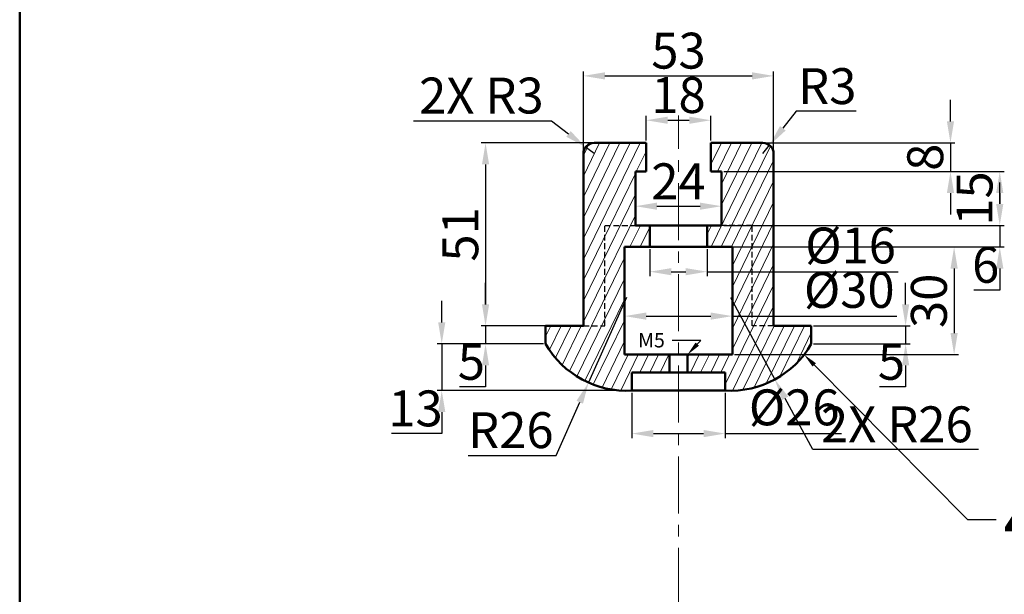
# Model space of a CAD drawing. Units: millimetres. Extents: x 147 to 984, y -369 to 435.
# Tile 2 of 10: x 147 to 422, y -208 to -48. Entities that reach past the tile are written whole.
import ezdxf
from ezdxf import colors
from ezdxf.entities.mleader import LeaderData, LeaderLine
from ezdxf.math import Vec2, Vec3

# ---------------------------------------------------------------- set-up
doc = ezdxf.new("R2010")
doc.units = ezdxf.units.MM
doc.header["$LTSCALE"] = 0.5
doc.linetypes.add('CENTER', pattern=[50.8, 31.75, -6.35, 6.35, -6.35])
doc.linetypes.add('HIDDEN', pattern=[9.525, 6.35, -3.175])
for name, color, linetype, lineweight in [('M-CNTR', 1, 'CENTER', 18), ('M-DIMS', 2, 'Continuous', 25), ('M-HATC', 8, 'Continuous', 18), ('M-HIDN', 3, 'HIDDEN', 25), ('M-OUTL', 7, 'Continuous', 50), ('M-TEXT', 7, 'Continuous', 25)]:
    doc.layers.add(name, color=color, linetype=linetype, lineweight=lineweight)
doc.styles.get("Standard").update_dxf_attribs({"font": 'arial.ttf'})
doc.dimstyles.new('ISO-25', dxfattribs={"dimtxt": 10, "dimasz": 6, "dimexe": 1.25, "dimexo": 0.625, "dimtad": 1, "dimtoh": 1, "dimdec": 0, "dimtxsty": 'Standard', "dimcen": 2.5, "dimadec": 0, "dimazin": 0, "dimtfac": 1, "dimtdec": 0, "dimtmove": 0, "dimatfit": 3, "dimfxl": 1, "dimarcsym": 0})

# ---------------------------------------------------------------- blocks, each defined once
blk = doc.blocks.new('*U94')
at = {"layer": 'M-CNTR', "color": 0, "transparency": 16777216}
blk.add_line((0, -186.27), (0, 51.67), dxfattribs=at)
blk = doc.blocks.new('*D95')
at = {"layer": 'Defpoints', "color": 0, "ltscale": 0.5, "transparency": 16777216}
for p in [(318.85, -100.29), (342.85, -100.29), (342.85, -100.29)]:
    blk.add_point(p, dxfattribs=at)
at = {"layer": 'M-DIMS', "color": 0, "lineweight": -2, "ltscale": 0.5, "transparency": 16777216}
for p, q in [((318.85, -99.67), (318.85, -99.04)), ((324.85, -100.29), (336.85, -100.29)), ((342.85, -99.67), (342.85, -99.04))]:
    blk.add_line(p, q, dxfattribs=at)
at = {"layer": 'M-DIMS', "color": 0, "ltscale": 0.5, "transparency": 16777216}
for points in [[(324.85, -99.29), (324.85, -101.29), (318.85, -100.29)], [(336.85, -99.29), (336.85, -101.29), (342.85, -100.29)]]:
    blk.add_solid(points, dxfattribs=at)
at = {"layer": 'M-DIMS', "color": 0, "ltscale": 0.5, "transparency": 16777216, "insert": (330.85, -94.65), "char_height": 10, "attachment_point": 5}
blk.add_mtext('24', dxfattribs=at)
blk = doc.blocks.new('*D96')
at = {"layer": 'Defpoints', "color": 0, "ltscale": 0.5, "transparency": 16777216}
for p in [(339.85, -76.35), (321.85, -82.65), (339.85, -82.65)]:
    blk.add_point(p, dxfattribs=at)
at = {"layer": 'M-DIMS', "color": 0, "lineweight": -2, "ltscale": 0.5, "transparency": 16777216}
for p, q in [((321.85, -82.03), (321.85, -75.1)), ((327.85, -76.35), (333.85, -76.35)), ((339.85, -82.03), (339.85, -75.1))]:
    blk.add_line(p, q, dxfattribs=at)
at = {"layer": 'M-DIMS', "color": 0, "ltscale": 0.5, "transparency": 16777216}
for points in [[(327.85, -75.35), (327.85, -77.35), (321.85, -76.35)], [(333.85, -75.35), (333.85, -77.35), (339.85, -76.35)]]:
    blk.add_solid(points, dxfattribs=at)
at = {"layer": 'M-DIMS', "color": 0, "ltscale": 0.5, "transparency": 16777216, "insert": (330.85, -70.62), "char_height": 10, "attachment_point": 5}
blk.add_mtext('18', dxfattribs=at)
blk = doc.blocks.new('*D97')
at = {"layer": 'Defpoints', "color": 0, "ltscale": 0.5, "transparency": 16777216}
for p in [(357.35, -63.98), (304.35, -85.65), (357.35, -85.65)]:
    blk.add_point(p, dxfattribs=at)
at = {"layer": 'M-DIMS', "color": 0, "lineweight": -2, "ltscale": 0.5, "transparency": 16777216}
for p, q in [((304.35, -85.03), (304.35, -62.73)), ((357.35, -85.03), (357.35, -62.73)), ((310.35, -63.98), (351.35, -63.98))]:
    blk.add_line(p, q, dxfattribs=at)
at = {"layer": 'M-DIMS', "color": 0, "ltscale": 0.5, "transparency": 16777216}
for points in [[(310.35, -62.98), (310.35, -64.98), (304.35, -63.98)], [(351.35, -62.98), (351.35, -64.98), (357.35, -63.98)]]:
    blk.add_solid(points, dxfattribs=at)
at = {"layer": 'M-DIMS', "color": 0, "ltscale": 0.5, "transparency": 16777216, "insert": (330.85, -58.25), "char_height": 10, "attachment_point": 5}
blk.add_mtext('53', dxfattribs=at)
blk = doc.blocks.new('*D99')
at = {"layer": 'Defpoints', "color": 0, "ltscale": 0.5, "transparency": 16777216}
for p in [(314.6, -82.65), (277.11, -133.65), (299.1, -133.65)]:
    blk.add_point(p, dxfattribs=at)
at = {"layer": 'M-DIMS', "color": 0, "lineweight": -2, "ltscale": 0.5, "transparency": 16777216}
for p, q in [((313.97, -82.65), (275.86, -82.65)), ((277.11, -88.65), (277.11, -127.65)), ((298.47, -133.65), (275.86, -133.65))]:
    blk.add_line(p, q, dxfattribs=at)
at = {"layer": 'M-DIMS', "color": 0, "ltscale": 0.5, "transparency": 16777216}
for points in [[(276.11, -88.65), (278.11, -88.65), (277.11, -82.65)], [(276.11, -127.65), (278.11, -127.65), (277.11, -133.65)]]:
    blk.add_solid(points, dxfattribs=at)
at = {"layer": 'M-DIMS', "color": 0, "ltscale": 0.5, "transparency": 16777216, "insert": (271.37, -108.15), "char_height": 10, "attachment_point": 5, "rotation": 90}
blk.add_mtext('51', dxfattribs=at)
blk = doc.blocks.new('*D100')
at = {"layer": 'Defpoints', "color": 0, "ltscale": 0.5, "transparency": 16777216}
for p in [(299.1, -133.65), (277.11, -138.65), (293.85, -138.65)]:
    blk.add_point(p, dxfattribs=at)
at = {"layer": 'M-DIMS', "color": 0, "lineweight": -2, "ltscale": 0.5, "transparency": 16777216}
for p, q in [((277.11, -127.65), (277.11, -121.65)), ((298.47, -133.65), (275.86, -133.65)), ((277.11, -133.65), (277.11, -138.65)), ((293.22, -138.65), (275.86, -138.65)), ((277.11, -144.65), (277.11, -150.65)), ((277.11, -150.65), (269.85, -150.65))]:
    blk.add_line(p, q, dxfattribs=at)
at = {"layer": 'M-DIMS', "color": 0, "ltscale": 0.5, "transparency": 16777216}
for points in [[(276.11, -127.65), (278.11, -127.65), (277.11, -133.65)], [(276.11, -144.65), (278.11, -144.65), (277.11, -138.65)]]:
    blk.add_solid(points, dxfattribs=at)
at = {"layer": 'M-DIMS', "color": 0, "ltscale": 0.5, "transparency": 16777216, "insert": (273.16, -144.94), "char_height": 10, "attachment_point": 5}
blk.add_mtext('5', dxfattribs=at)
blk = doc.blocks.new('*D101')
at = {"layer": 'Defpoints', "color": 0, "ltscale": 0.5, "transparency": 16777216}
for p in [(293.85, -138.65), (264.91, -151.65), (330.85, -151.65)]:
    blk.add_point(p, dxfattribs=at)
at = {"layer": 'M-DIMS', "color": 0, "lineweight": -2, "ltscale": 0.5, "transparency": 16777216}
for p, q in [((264.91, -132.65), (264.91, -126.65)), ((293.22, -138.65), (263.66, -138.65)), ((264.91, -138.65), (264.91, -151.65)), ((330.22, -151.65), (263.66, -151.65)), ((264.91, -157.65), (264.91, -163.65)), ((264.91, -163.65), (250.9, -163.65))]:
    blk.add_line(p, q, dxfattribs=at)
at = {"layer": 'M-DIMS', "color": 0, "ltscale": 0.5, "transparency": 16777216}
for points in [[(263.91, -132.65), (265.91, -132.65), (264.91, -138.65)], [(263.91, -157.65), (265.91, -157.65), (264.91, -151.65)]]:
    blk.add_solid(points, dxfattribs=at)
at = {"layer": 'M-DIMS', "color": 0, "ltscale": 0.5, "transparency": 16777216, "insert": (257.6, -157.92), "char_height": 10, "attachment_point": 5}
blk.add_mtext('13', dxfattribs=at)
blk = doc.blocks.new('*D102')
at = {"layer": 'Defpoints', "color": 0, "ltscale": 0.5, "transparency": 16777216}
for p in [(322.85, -111.65), (338.85, -111.65), (338.85, -118.54)]:
    blk.add_point(p, dxfattribs=at)
at = {"layer": 'M-DIMS', "color": 0, "lineweight": -2, "ltscale": 0.5, "transparency": 16777216}
for p, q in [((322.85, -112.28), (322.85, -119.79)), ((338.85, -112.28), (338.85, -119.79)), ((328.85, -118.54), (332.85, -118.54)), ((338.85, -118.54), (392, -118.54))]:
    blk.add_line(p, q, dxfattribs=at)
at = {"layer": 'M-DIMS', "color": 0, "ltscale": 0.5, "transparency": 16777216}
for points in [[(328.85, -117.54), (328.85, -119.54), (322.85, -118.54)], [(332.85, -117.54), (332.85, -119.54), (338.85, -118.54)]]:
    blk.add_solid(points, dxfattribs=at)
at = {"layer": 'M-DIMS', "color": 0, "ltscale": 0.5, "transparency": 16777216, "insert": (378.77, -112.53), "char_height": 10, "attachment_point": 5}
blk.add_mtext('%%C16', dxfattribs=at)
blk = doc.blocks.new('*D103')
at = {"layer": 'Defpoints', "color": 0, "ltscale": 0.5, "transparency": 16777216}
for p in [(315.85, -126.65), (345.85, -126.65), (345.85, -130.92)]:
    blk.add_point(p, dxfattribs=at)
at = {"layer": 'M-DIMS', "color": 0, "lineweight": -2, "ltscale": 0.5, "transparency": 16777216}
for p, q in [((315.85, -127.28), (315.85, -132.17)), ((345.85, -127.28), (345.85, -132.17)), ((321.85, -130.92), (339.85, -130.92)), ((345.85, -130.92), (391.62, -130.92))]:
    blk.add_line(p, q, dxfattribs=at)
at = {"layer": 'M-DIMS', "color": 0, "ltscale": 0.5, "transparency": 16777216}
for points in [[(321.85, -129.92), (321.85, -131.92), (315.85, -130.92)], [(339.85, -129.92), (339.85, -131.92), (345.85, -130.92)]]:
    blk.add_solid(points, dxfattribs=at)
at = {"layer": 'M-DIMS', "color": 0, "ltscale": 0.5, "transparency": 16777216, "insert": (378.41, -124.91), "char_height": 10, "attachment_point": 5}
blk.add_mtext('%%C30', dxfattribs=at)
blk = doc.blocks.new('*D104')
at = {"layer": 'Defpoints', "color": 0, "ltscale": 0.5, "transparency": 16777216}
for p in [(317.85, -151.65), (343.85, -151.65), (343.85, -163.65)]:
    blk.add_point(p, dxfattribs=at)
at = {"layer": 'M-DIMS', "color": 0, "lineweight": -2, "ltscale": 0.5, "transparency": 16777216}
for p, q in [((317.85, -152.28), (317.85, -164.9)), ((343.85, -152.28), (343.85, -164.9)), ((323.85, -163.65), (337.85, -163.65)), ((343.85, -163.65), (376.29, -163.65))]:
    blk.add_line(p, q, dxfattribs=at)
at = {"layer": 'M-DIMS', "color": 0, "ltscale": 0.5, "transparency": 16777216}
for points in [[(323.85, -162.65), (323.85, -164.65), (317.85, -163.65)], [(337.85, -162.65), (337.85, -164.65), (343.85, -163.65)]]:
    blk.add_solid(points, dxfattribs=at)
at = {"layer": 'M-DIMS', "color": 0, "ltscale": 0.5, "transparency": 16777216, "insert": (363.07, -157.64), "char_height": 10, "attachment_point": 5}
blk.add_mtext('%%C26', dxfattribs=at)
blk = doc.blocks.new('*D105')
at = {"layer": 'Defpoints', "color": 0, "ltscale": 0.5, "transparency": 16777216}
for p in [(316.39, -125.7), (305.79, -149.44)]:
    blk.add_point(p, dxfattribs=at)
at = {"layer": 'M-DIMS', "color": 0, "lineweight": -2, "ltscale": 0.5, "transparency": 16777216}
for p, q in [((316.39, -125.7), (305.79, -149.44)), ((296.73, -169.72), (303.34, -154.92)), ((272.22, -169.72), (296.73, -169.72))]:
    blk.add_line(p, q, dxfattribs=at)
at = {"layer": 'M-DIMS', "color": 0, "ltscale": 0.5, "transparency": 16777216}
blk.add_solid([(302.43, -154.51), (304.25, -155.32), (305.79, -149.44)], dxfattribs=at)
at = {"layer": 'M-DIMS', "color": 0, "ltscale": 0.5, "transparency": 16777216, "insert": (284.16, -163.99), "char_height": 10, "attachment_point": 5}
blk.add_mtext('R26', dxfattribs=at)
blk = doc.blocks.new('*D106')
at = {"layer": 'Defpoints', "color": 0, "ltscale": 0.5, "transparency": 16777216}
for p in [(356.2, -83.3), (354.35, -85.65)]:
    blk.add_point(p, dxfattribs=at)
at = {"layer": 'M-DIMS', "color": 0, "lineweight": -2, "ltscale": 0.5, "transparency": 16777216}
for p, q in [((363.61, -73.86), (359.91, -78.58)), ((380.37, -73.86), (363.61, -73.86)), ((354.35, -85.65), (356.2, -83.3))]:
    blk.add_line(p, q, dxfattribs=at)
at = {"layer": 'M-DIMS', "color": 0, "ltscale": 0.5, "transparency": 16777216}
blk.add_solid([(359.12, -77.96), (360.69, -79.2), (356.2, -83.3)], dxfattribs=at)
at = {"layer": 'M-DIMS', "color": 0, "ltscale": 0.5, "transparency": 16777216, "insert": (372.3, -68.13), "char_height": 10, "attachment_point": 5}
blk.add_mtext('R3', dxfattribs=at)
blk = doc.blocks.new('*D107')
at = {"layer": 'Defpoints', "color": 0, "ltscale": 0.5, "transparency": 16777216}
for p in [(347.1, -82.65), (342.85, -90.65), (406.6, -90.65)]:
    blk.add_point(p, dxfattribs=at)
at = {"layer": 'M-DIMS', "color": 0, "lineweight": -2, "ltscale": 0.5, "transparency": 16777216}
for p, q in [((406.6, -76.65), (406.6, -70.65)), ((347.72, -82.65), (407.85, -82.65)), ((406.6, -82.65), (406.6, -90.65)), ((343.47, -90.65), (407.85, -90.65)), ((406.6, -96.65), (406.6, -102.65))]:
    blk.add_line(p, q, dxfattribs=at)
at = {"layer": 'M-DIMS', "color": 0, "ltscale": 0.5, "transparency": 16777216}
for points in [[(405.6, -76.65), (407.6, -76.65), (406.6, -82.65)], [(405.6, -96.65), (407.6, -96.65), (406.6, -90.65)]]:
    blk.add_solid(points, dxfattribs=at)
at = {"layer": 'M-DIMS', "color": 0, "ltscale": 0.5, "transparency": 16777216, "insert": (400.87, -86.65), "char_height": 10, "attachment_point": 5, "rotation": 90}
blk.add_mtext('8', dxfattribs=at)
blk = doc.blocks.new('*D108')
at = {"layer": 'Defpoints', "color": 0, "ltscale": 0.5, "transparency": 16777216}
for p in [(342.85, -90.65), (342.85, -105.65), (420.33, -105.65)]:
    blk.add_point(p, dxfattribs=at)
at = {"layer": 'M-DIMS', "color": 0, "lineweight": -2, "ltscale": 0.5, "transparency": 16777216}
for p, q in [((343.47, -90.65), (421.58, -90.65)), ((420.33, -96.65), (420.33, -99.65)), ((343.47, -105.65), (421.58, -105.65))]:
    blk.add_line(p, q, dxfattribs=at)
at = {"layer": 'M-DIMS', "color": 0, "ltscale": 0.5, "transparency": 16777216}
for points in [[(419.33, -96.65), (421.33, -96.65), (420.33, -90.65)], [(419.33, -99.65), (421.33, -99.65), (420.33, -105.65)]]:
    blk.add_solid(points, dxfattribs=at)
at = {"layer": 'M-DIMS', "color": 0, "ltscale": 0.5, "transparency": 16777216, "insert": (414.6, -98.15), "char_height": 10, "attachment_point": 5, "rotation": 90}
blk.add_mtext('15', dxfattribs=at)
blk = doc.blocks.new('*D109')
at = {"layer": 'Defpoints', "color": 0, "ltscale": 0.5, "transparency": 16777216}
for p in [(342.85, -105.65), (342.85, -111.65), (420.33, -111.65)]:
    blk.add_point(p, dxfattribs=at)
at = {"layer": 'M-DIMS', "color": 0, "lineweight": -2, "ltscale": 0.5, "transparency": 16777216}
for p, q in [((420.33, -99.65), (420.33, -93.65)), ((343.47, -105.65), (421.58, -105.65)), ((420.33, -105.65), (420.33, -111.65)), ((343.47, -111.65), (421.58, -111.65)), ((420.33, -117.65), (420.33, -123.65)), ((420.33, -123.65), (413.11, -123.65))]:
    blk.add_line(p, q, dxfattribs=at)
at = {"layer": 'M-DIMS', "color": 0, "ltscale": 0.5, "transparency": 16777216}
for points in [[(419.33, -99.65), (421.33, -99.65), (420.33, -105.65)], [(419.33, -117.65), (421.33, -117.65), (420.33, -111.65)]]:
    blk.add_solid(points, dxfattribs=at)
at = {"layer": 'M-DIMS', "color": 0, "ltscale": 0.5, "transparency": 16777216, "insert": (416.41, -117.92), "char_height": 10, "attachment_point": 5}
blk.add_mtext('6', dxfattribs=at)
blk = doc.blocks.new('*D110')
at = {"layer": 'Defpoints', "color": 0, "ltscale": 0.5, "transparency": 16777216}
for p in [(345.85, -111.65), (345.85, -141.65), (407.62, -141.65)]:
    blk.add_point(p, dxfattribs=at)
at = {"layer": 'M-DIMS', "color": 0, "lineweight": -2, "ltscale": 0.5, "transparency": 16777216}
for p, q in [((346.47, -111.65), (408.87, -111.65)), ((407.62, -117.65), (407.62, -135.65)), ((346.47, -141.65), (408.87, -141.65))]:
    blk.add_line(p, q, dxfattribs=at)
at = {"layer": 'M-DIMS', "color": 0, "ltscale": 0.5, "transparency": 16777216}
for points in [[(406.62, -117.65), (408.62, -117.65), (407.62, -111.65)], [(406.62, -135.65), (408.62, -135.65), (407.62, -141.65)]]:
    blk.add_solid(points, dxfattribs=at)
at = {"layer": 'M-DIMS', "color": 0, "ltscale": 0.5, "transparency": 16777216, "insert": (401.89, -126.65), "char_height": 10, "attachment_point": 5, "rotation": 90}
blk.add_mtext('30', dxfattribs=at)
blk = doc.blocks.new('*D111')
at = {"layer": 'Defpoints', "color": 0, "ltscale": 0.5, "transparency": 16777216}
for p in [(367.85, -133.65), (367.85, -138.65), (394.11, -138.65)]:
    blk.add_point(p, dxfattribs=at)
at = {"layer": 'M-DIMS', "color": 0, "lineweight": -2, "ltscale": 0.5, "transparency": 16777216}
for p, q in [((394.11, -127.65), (394.11, -121.65)), ((368.47, -133.65), (395.36, -133.65)), ((394.11, -133.65), (394.11, -138.65)), ((368.47, -138.65), (395.36, -138.65)), ((394.11, -144.65), (394.11, -150.65)), ((394.11, -150.65), (386.86, -150.65))]:
    blk.add_line(p, q, dxfattribs=at)
at = {"layer": 'M-DIMS', "color": 0, "ltscale": 0.5, "transparency": 16777216}
for points in [[(393.11, -127.65), (395.11, -127.65), (394.11, -133.65)], [(393.11, -144.65), (395.11, -144.65), (394.11, -138.65)]]:
    blk.add_solid(points, dxfattribs=at)
at = {"layer": 'M-DIMS', "color": 0, "ltscale": 0.5, "transparency": 16777216, "insert": (390.17, -144.94), "char_height": 10, "attachment_point": 5}
blk.add_mtext('5', dxfattribs=at)
blk = doc.blocks.new('*D180')
at = {"layer": 'Defpoints', "color": 0, "ltscale": 0.5, "transparency": 16777216}
for p in [(345.31, -125.7), (357.69, -148.56)]:
    blk.add_point(p, dxfattribs=at)
at = {"layer": 'M-DIMS', "color": 0, "lineweight": -2, "ltscale": 0.5, "transparency": 16777216}
for p, q in [((345.31, -125.7), (357.69, -148.56)), ((368.27, -168.09), (360.55, -153.83)), ((414.44, -168.09), (368.27, -168.09))]:
    blk.add_line(p, q, dxfattribs=at)
at = {"layer": 'M-DIMS', "color": 0, "ltscale": 0.5, "transparency": 16777216}
blk.add_solid([(361.43, -153.36), (359.67, -154.31), (357.69, -148.56)], dxfattribs=at)
at = {"layer": 'M-DIMS', "color": 0, "ltscale": 0.5, "transparency": 16777216, "insert": (391.67, -162.36), "char_height": 10, "attachment_point": 5}
blk.add_mtext('2X R26', dxfattribs=at)
blk = doc.blocks.new('*D181')
at = {"layer": 'Defpoints', "color": 0, "ltscale": 0.5, "transparency": 16777216}
for p in [(304.97, -83.82), (307.35, -85.65)]:
    blk.add_point(p, dxfattribs=at)
at = {"layer": 'M-DIMS', "color": 0, "lineweight": -2, "ltscale": 0.5, "transparency": 16777216}
for p, q in [((257.06, -76.5), (295.47, -76.5)), ((295.47, -76.5), (300.22, -80.16)), ((307.35, -85.65), (304.97, -83.82))]:
    blk.add_line(p, q, dxfattribs=at)
at = {"layer": 'M-DIMS', "color": 0, "ltscale": 0.5, "transparency": 16777216}
blk.add_solid([(300.83, -79.37), (299.61, -80.95), (304.97, -83.82)], dxfattribs=at)
at = {"layer": 'M-DIMS', "color": 0, "ltscale": 0.5, "transparency": 16777216, "insert": (275.95, -70.76), "char_height": 10, "attachment_point": 5}
blk.add_mtext('2X R3', dxfattribs=at)

msp = doc.modelspace()

# ---------------------------------------------------------------- hatches: boundary and pattern name
at = {"layer": 'M-HATC', "ltscale": 0.5}
h = msp.add_hatch(dxfattribs=at)
h.set_pattern_fill('ANSI31', color=256, scale=0.8, angle=199)
h.set_pattern_definition([(244, (-217.7436, 170.283), (2.282937, -1.113463), [])])
h.paths.add_polyline_path([(318.8467, -90.6547), (321.8467, -90.6547), (321.8467, -82.6547), (307.3467, -82.6547, 0.41421356), (304.3467, -85.6547), (304.3467, -133.6547), (310.3467, -133.6547), (310.3467, -105.6547), (318.8467, -105.6547)])
h.paths.add_polyline_path([(357.3467, -85.6547, 0.41421356), (354.3467, -82.6547), (339.8467, -82.6547), (339.8467, -90.6547), (342.8467, -90.6547), (342.8467, -105.6547), (351.3467, -105.6547), (351.3467, -133.6547), (357.3467, -133.6547)])
h.paths.add_polyline_path([(315.8467, -111.6547), (322.8467, -111.6547), (322.8467, -105.6547), (318.8467, -105.6547), (310.3467, -105.6547), (310.3467, -133.6547), (304.3467, -133.6547), (293.8467, -133.6547), (293.8467, -138.6547, 0.28354997), (317.8467, -151.6547), (317.8467, -146.6547), (328.3467, -146.6547), (328.3467, -141.6547), (315.8467, -141.6547)])
h.paths.add_polyline_path([(367.8467, -138.6547), (367.8467, -133.6547), (357.3467, -133.6547), (351.3467, -133.6547), (351.3467, -105.6547), (342.8467, -105.6547), (338.8467, -105.6547), (338.8467, -111.6547), (345.8467, -111.6547), (345.8467, -141.6547), (333.3467, -141.6547), (333.3467, -146.6547), (343.8467, -146.6547), (343.8467, -151.6547, 0.28354997)])

# ---------------------------------------------------------------- linework, layer by layer
at = {"layer": 'M-HIDN', "ltscale": 0.5}
for p, q in [((310.3467, -133.6547), (310.3467, -105.6547)), ((310.3467, -105.6547), (318.8467, -105.6547)), ((351.3467, -105.6547), (342.8467, -105.6547)), ((351.3467, -133.6547), (351.3467, -105.6547)), ((304.3467, -133.6547), (310.3467, -133.6547)), ((357.3467, -133.6547), (351.3467, -133.6547))]:
    msp.add_line(p, q, dxfattribs=at)
at = {"layer": 'M-OUTL', "ltscale": 0.5}
for p, q in [((321.8467, -82.6547), (307.3467, -82.6547)), ((321.8467, -90.6547), (321.8467, -82.6547)), ((339.8467, -90.6547), (339.8467, -82.6547)), ((339.8467, -82.6547), (354.3467, -82.6547)), ((304.3467, -85.6547), (304.3467, -133.6547)), ((357.3467, -85.6547), (357.3467, -133.6547)), ((318.8467, -105.6547), (318.8467, -90.6547)), ((318.8467, -90.6547), (321.8467, -90.6547)), ((342.8467, -90.6547), (339.8467, -90.6547)), ((342.8467, -105.6547), (342.8467, -90.6547)), ((318.8467, -105.6547), (342.8467, -105.6547)), ((322.8467, -105.6547), (338.8467, -105.6547)), ((322.8467, -111.6547), (322.8467, -105.6547)), ((338.8467, -105.6547), (338.8467, -111.6547)), ((315.8467, -111.6547), (345.8467, -111.6547)), ((315.8467, -141.6547), (315.8467, -111.6547)), ((338.8467, -111.6547), (322.8467, -111.6547)), ((345.8467, -111.6547), (345.8467, -141.6547)), ((304.3467, -133.6547), (293.8467, -133.6547)), ((293.8467, -133.6547), (293.8467, -138.6547)), ((357.3467, -133.6547), (367.8467, -133.6547)), ((367.8467, -133.6547), (367.8467, -138.6547)), ((345.8467, -141.6547), (315.8467, -141.6547)), ((328.3467, -141.6547), (333.3467, -141.6547)), ((328.3467, -146.6547), (328.3467, -141.6547)), ((333.3467, -141.6547), (333.3467, -146.6547)), ((317.8467, -146.6547), (343.8467, -146.6547)), ((317.8467, -151.6547), (317.8467, -146.6547)), ((333.3467, -146.6547), (328.3467, -146.6547)), ((343.8467, -146.6547), (343.8467, -151.6547)), ((343.8467, -151.6547), (317.8467, -151.6547))]:
    msp.add_line(p, q, dxfattribs=at)
msp.add_lwpolyline([(147.3511, 435.3078), (984.0884, 435.3078), (984.0884, -369.4968), (147.3511, -369.4968)], close=True, dxfattribs=at)
for centre, radius, start, end in [((307.3467, -85.6547), 3, 90, 180), ((354.3467, -85.6547), 3, 0, 90), ((316.387, -125.6957), 26, 209.895705, 273.218438), ((345.3064, -125.6957), 26, 266.781562, 330.104295)]:
    msp.add_arc(centre, radius, start, end, dxfattribs=at)

# ---------------------------------------------------------------- block references
at = {"layer": 'M-CNTR'}
msp.add_blockref('*U94', (330.8467, -126.6547), dxfattribs=at)

# ---------------------------------------------------------------- dimensions: what is measured, and where the dimension line sits
at = {"layer": 'M-DIMS', "ltscale": 0.5}
for base, p1, p2, picture, middle in [((357.3467, -63.9839), (304.3467, -85.6547), (357.3467, -85.6547), '*D97', (330.8467, -58.2498)), ((339.8467, -76.3543), (321.8467, -82.6547), (339.8467, -82.6547), '*D96', (330.8467, -70.6235)), ((342.8467, -100.2909), (318.8467, -100.2909), (342.8467, -100.2909), '*D95', (330.8467, -94.6455))]:
    dim = msp.add_linear_dim(base=base, p1=p1, p2=p2, dimstyle='ISO-25', override={"dimclrd": 0, "dimclre": 0, "dimclrt": 0}, dxfattribs=at)
    dim.commit()
    dim.dimension.update_dxf_attribs({"geometry": picture, "text_midpoint": middle})
for center, mpoint, picture, middle in [((307.3467, -85.6547), (304.9707, -83.8232), '*D181', (275.9499, -70.7631)), ((345.3064, -125.6957), (357.6901, -148.5571), '*D180', (391.6671, -162.3566))]:
    dim = msp.add_radius_dim(center=center, mpoint=mpoint, text='2X <>', dimstyle='ISO-25', override={"dimdec": 0, "dimlfac": 1, "dimrnd": 0, "dimzin": 0, "dimdsep": 46, "dimlunit": 2}, dxfattribs=at)
    dim.commit()
    dim.dimension.update_dxf_attribs({"geometry": picture, "text_midpoint": middle})
for center, mpoint, picture, middle in [((354.3467, -85.6547), (356.2003, -83.2958), '*D106', (372.3023, -68.1262)), ((316.387, -125.6957), (305.7866, -149.4366), '*D105', (284.1617, -163.9874))]:
    dim = msp.add_radius_dim(center=center, mpoint=mpoint, dimstyle='ISO-25', override={"dimclrd": 0, "dimclre": 0, "dimclrt": 0}, dxfattribs=at)
    dim.commit()
    dim.dimension.update_dxf_attribs({"geometry": picture, "text_midpoint": middle})
for base, p1, p2, picture, middle in [((406.604, -90.6547), (347.0967, -82.6547), (342.8467, -90.6547), '*D107', (400.8733, -86.6547)), ((277.1051, -133.6547), (314.5967, -82.6547), (299.0967, -133.6547), '*D99', (271.3744, -108.1547)), ((420.333, -105.6547), (342.8467, -90.6547), (342.8467, -105.6547), '*D108', (414.6023, -98.1547)), ((420.333, -111.6547), (342.8467, -105.6547), (342.8467, -111.6547), '*D109', (416.4065, -117.924)), ((407.624, -141.6547), (345.8467, -111.6547), (345.8467, -141.6547), '*D110', (401.8899, -126.6547)), ((277.1051, -138.6547), (299.0967, -133.6547), (293.8467, -138.6547), '*D100', (273.165, -144.9444)), ((394.1106, -138.6547), (367.8467, -133.6547), (367.8467, -138.6547), '*D111', (390.1705, -144.9444)), ((264.9133, -151.6547), (293.8467, -138.6547), (330.8467, -151.6547), '*D101', (257.5966, -157.9206))]:
    dim = msp.add_linear_dim(base=base, p1=p1, p2=p2, angle=90, dimstyle='ISO-25', override={"dimclrd": 0, "dimclre": 0, "dimclrt": 0}, dxfattribs=at)
    dim.commit()
    dim.dimension.update_dxf_attribs({"geometry": picture, "text_midpoint": middle})
for base, p1, p2, picture, middle in [((338.8467, -118.5364), (322.8467, -111.6547), (338.8467, -111.6547), '*D102', (378.7727, -118.5364)), ((345.8467, -130.9176), (315.8467, -126.6547), (345.8467, -126.6547), '*D103', (378.4121, -130.9176))]:
    dim = msp.add_linear_dim(base=base, p1=p1, p2=p2, text='%%C<>', dimstyle='ISO-25', override={"dimclrd": 0, "dimclre": 0, "dimclrt": 0}, dxfattribs=at)
    dim.commit()
    dim.dimension.update_dxf_attribs({"geometry": picture, "text_midpoint": middle, "dimtype": 160})
dim = msp.add_linear_dim(base=(343.8467, -163.6529), p1=(317.8467, -151.6547), p2=(343.8467, -151.6547), text='%%C<>', dimstyle='ISO-25', override={"dimclrd": 0, "dimclre": 0, "dimclrt": 0}, dxfattribs=at)
dim.commit()
dim.dimension.update_dxf_attribs({"geometry": '*D104', "text_midpoint": (363.0706, -157.6425)})

# ---------------------------------------------------------------- leaders
at = {"layer": 'M-TEXT', "ltscale": 0.5}
ml = msp.add_multileader_mtext('Standard', dxfattribs=at)
ml.set_content('M5', color=256)
ml.set_leader_properties()
ml.build(insert=Vec2(0, 0))
ctx = ml.context
ctx.base_point, ctx.plane_origin = Vec3(317.9243, -137.676), Vec3(333.3467, -141.6547)
ctx.text_align_type = 2
notes = []
notes.append((ctx, [(0, (1, 1, 0), (337.0484, -137.676), (-1, 0), 8, [(0, [(333.3467, -141.6547)], 0, [])])]))
ctx.mtext.insert, ctx.mtext.alignment, ctx.mtext.flow_direction = Vec3(327.0484, -135.6419), 3, 5
ml = msp.add_multileader_mtext('Standard', dxfattribs=at)
ml.set_content('4', color=256)
ml.set_leader_properties()
ml.build(insert=Vec2(0, 0))
ctx = ml.context
ctx.base_point, ctx.char_height, ctx.plane_origin = Vec3(419.374, -187.5359), 15, Vec3(365.8323, -141.6547)
notes.append((ctx, [(0, (1, 1, 0), (411.374, -187.5359), (1, 0), 8, [(0, [(365.8323, -141.6547)], 0, [])])]))
ctx.mtext.insert, ctx.mtext.flow_direction = Vec3(421.374, -180.0359), 5
for ctx, leaders in notes:
    for number, flags, end, landing, length, lines in leaders:
        leader = LeaderData()
        leader.index, (leader.has_last_leader_line, leader.has_dogleg_vector, leader.attachment_direction) = number, flags
        leader.last_leader_point, leader.dogleg_vector, leader.dogleg_length = Vec3(end), Vec3(landing), length
        for number, points, colour, breaks in lines:
            line = LeaderLine()
            line.index, line.vertices, line.color, line.breaks = number, Vec3.list(points), colors.encode_raw_color(colour), breaks
            leader.lines.append(line)
        ctx.leaders.append(leader)

doc.saveas('drawing.dxf')
